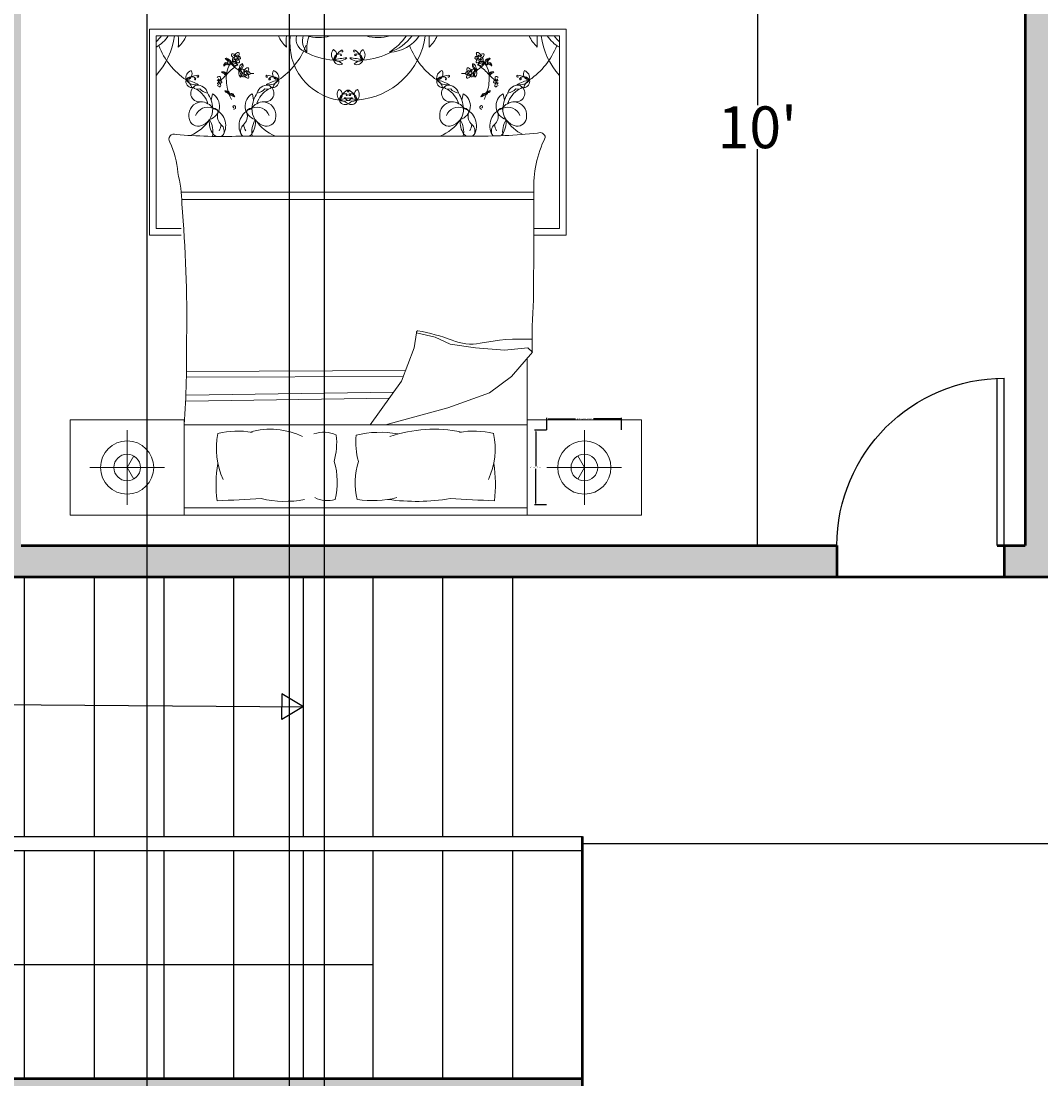
# Model space of a CAD drawing. Units: inches. Extents: x -22 to 470, y -437 to 97.
# Tile 6 of 9: x 88 to 235, y -192 to -41. Entities that reach past the tile are written whole.
import ezdxf

# ---------------------------------------------------------------- set-up
doc = ezdxf.new("R2010")
doc.units = ezdxf.units.IN
doc.header["$MEASUREMENT"] = 0
for name, color, linetype, lineweight in [('A-ANNO-DIMS', 2, 'Continuous', 18), ('A-DOOR', 4, 'Continuous', 25), ('A-FLOR-STRS', 7, 'Continuous', 25), ('A-FURN', 8, 'Continuous', 18), ('A-WALL', 7, 'Continuous', 50), ('A-WALL-PATT', 8, 'Continuous', 13)]:
    doc.layers.add(name, color=color, linetype=linetype, lineweight=lineweight)
doc.styles.get("Standard").update_dxf_attribs({"font": 'arial.ttf'})
doc.dimstyles.get("Standard").update_dxf_attribs({"dimtxt": 0.18, "dimasz": 0.18, "dimexe": 0.18, "dimexo": 0.0625, "dimgap": 0.09, "dimtad": 0, "dimtih": 1, "dimtoh": 1, "dimdec": 0, "dimzin": 0, "dimdsep": 46, "dimlunit": 3, "dimtxsty": 'Standard', "dimcen": 0.09, "dimadec": 0, "dimazin": 0, "dimtfac": 1, "dimtdec": 0, "dimtofl": 0, "dimtmove": 0, "dimatfit": 3, "dimfxl": 1, "dimtolj": 1, "dimtzin": 0, "dimarcsym": 0})

# ---------------------------------------------------------------- blocks, each defined once
blk = doc.blocks.new('*D6')
at = {"layer": 'A-ANNO-DIMS', "color": 0, "lineweight": -2, "transparency": 16777216}
for p, q in [((194.01, 4.06), (194.01, -52.6)), ((194.07, 4.24), (194.19, 4.24)), ((194.01, -115.58), (194.01, -58.91)), ((194.07, -115.76), (194.19, -115.76))]:
    blk.add_line(p, q, dxfattribs=at)
at = {"layer": 'A-ANNO-DIMS', "color": 0, "transparency": 16777216}
for points in [[(193.98, 4.06), (194.04, 4.06), (194.01, 4.24)], [(193.98, -115.58), (194.04, -115.58), (194.01, -115.76)]]:
    blk.add_solid(points, dxfattribs=at)
at = {"layer": 'Defpoints', "color": 0, "transparency": 16777216}
for p in [(194.01, 4.24), (194.01, 4.24), (194.01, -115.76)]:
    blk.add_point(p, dxfattribs=at)
at = {"layer": 'A-ANNO-DIMS', "color": 0, "transparency": 16777216, "insert": (194.01, -55.76), "char_height": 6, "attachment_point": 5}
blk.add_mtext("\\A1;10'", dxfattribs=at)
blk = doc.blocks.new('*D12')
at = {"layer": 'A-ANNO-DIMS', "color": 0, "lineweight": -2, "transparency": 16777216}
for p, q in [((168.92, -159.44), (168.92, -158.33)), ((169.1, -158.51), (240.81, -158.51)), ((332.74, -158.51), (261.03, -158.51)), ((332.92, -158.44), (332.92, -158.33))]:
    blk.add_line(p, q, dxfattribs=at)
at = {"layer": 'A-ANNO-DIMS', "color": 0, "transparency": 16777216}
for points in [[(169.1, -158.48), (169.1, -158.54), (168.92, -158.51)], [(332.74, -158.48), (332.74, -158.54), (332.92, -158.51)]]:
    blk.add_solid(points, dxfattribs=at)
at = {"layer": 'Defpoints', "color": 0, "transparency": 16777216}
for p in [(332.92, -158.51), (332.92, -158.51), (168.92, -159.51)]:
    blk.add_point(p, dxfattribs=at)
at = {"layer": 'A-ANNO-DIMS', "color": 0, "transparency": 16777216, "insert": (250.92, -158.51), "char_height": 6, "attachment_point": 5}
blk.add_mtext('\\A1;13\'-8"', dxfattribs=at)
blk = doc.blocks.new('DOOR-SWING-24')
for p, q in [((23, 24), (23, 0)), ((24, 24), (24, 0))]:
    blk.add_line(p, q)
blk.add_arc((24, 24), 24, 180, 270)
blk = doc.blocks.new('BEDSIDE-LAMP-LARGE')
for p, q in [((5.35, 10.71), (5.35, 0)), ((10.71, 5.36), (0, 5.36))]:
    blk.add_line(p, q)
for points in [[(5.35, 5.36), (6.31, 7.01)], [(5.35, 5.36), (6.31, 3.7)]]:
    blk.add_lwpolyline(points)
for radius in [3.82, 1.91]:
    blk.add_circle((5.35, 5.36), radius)
blk = doc.blocks.new('*D51')
at = {"layer": 'A-ANNO-DIMS', "color": 0, "lineweight": -2, "transparency": 16777216}
for p, q in [((163.84, -99.14), (163.84, -97.42)), ((164.02, -97.6), (167.91, -97.6)), ((174.37, -97.6), (170.49, -97.6)), ((174.55, -99.14), (174.55, -97.42))]:
    blk.add_line(p, q, dxfattribs=at)
at = {"layer": 'A-ANNO-DIMS', "color": 0, "transparency": 16777216}
for points in [[(164.02, -97.57), (164.02, -97.63), (163.84, -97.6)], [(174.37, -97.57), (174.37, -97.63), (174.55, -97.6)]]:
    blk.add_solid(points, dxfattribs=at)
at = {"layer": 'Defpoints', "color": 0, "transparency": 16777216}
for p in [(163.84, -97.6), (163.84, -99.21), (174.55, -99.21)]:
    blk.add_point(p, dxfattribs=at)
at = {"layer": 'A-ANNO-DIMS', "color": 0, "transparency": 16777216, "insert": (169.2, -97.6), "char_height": 0.18, "attachment_point": 5}
blk.add_mtext('\\A1;LAMP 0\'-10 1/2" TYP.', dxfattribs=at)
blk = doc.blocks.new('*D52')
at = {"layer": 'A-ANNO-DIMS', "color": 0, "lineweight": -2, "transparency": 16777216}
for p, q in [((163.78, -99.21), (162.06, -99.21)), ((162.24, -99.39), (162.24, -104.38)), ((162.24, -109.74), (162.24, -104.74)), ((163.78, -109.92), (162.06, -109.92))]:
    blk.add_line(p, q, dxfattribs=at)
at = {"layer": 'A-ANNO-DIMS', "color": 0, "transparency": 16777216}
for points in [[(162.21, -99.39), (162.27, -99.39), (162.24, -99.21)], [(162.21, -109.74), (162.27, -109.74), (162.24, -109.92)]]:
    blk.add_solid(points, dxfattribs=at)
at = {"layer": 'Defpoints', "color": 0, "transparency": 16777216}
for p in [(163.84, -99.21), (162.24, -109.92), (163.84, -109.92)]:
    blk.add_point(p, dxfattribs=at)
at = {"layer": 'A-ANNO-DIMS', "color": 0, "transparency": 16777216, "insert": (162.24, -104.56), "char_height": 0.18, "attachment_point": 5}
blk.add_mtext('\\A1;0\'-10 1/2" TYP.', dxfattribs=at)
blk = doc.blocks.new('*D79')
at = {"layer": 'A-ANNO-DIMS', "color": 0, "lineweight": -2, "transparency": 16777216}
for p, q in [((61.08, -228.48), (61.08, 40.87)), ((61.26, 40.69), (93.66, 40.69)), ((126.72, 40.69), (94.32, 40.69)), ((126.9, -228.48), (126.9, 40.87))]:
    blk.add_line(p, q, dxfattribs=at)
at = {"layer": 'A-ANNO-DIMS', "color": 0, "transparency": 16777216}
for points in [[(61.26, 40.72), (61.26, 40.66), (61.08, 40.69)], [(126.72, 40.72), (126.72, 40.66), (126.9, 40.69)]]:
    blk.add_solid(points, dxfattribs=at)
at = {"layer": 'Defpoints', "color": 0, "transparency": 16777216}
for p in [(126.9, 40.69), (61.08, -228.55), (126.9, -228.55)]:
    blk.add_point(p, dxfattribs=at)
at = {"layer": 'A-ANNO-DIMS', "color": 0, "transparency": 16777216, "insert": (93.99, 40.69), "char_height": 0.18, "attachment_point": 5}
blk.add_mtext('\\A1;5\'-6"', dxfattribs=at)
blk = doc.blocks.new('*D84')
at = {"layer": 'A-ANNO-DIMS', "color": 0, "lineweight": -2, "transparency": 16777216}
for p, q in [((106.48, -369.14), (106.48, 40.87)), ((106.66, 40.69), (118.66, 40.69)), ((131.74, 40.69), (119.74, 40.69)), ((131.92, -388.69), (131.92, 40.87))]:
    blk.add_line(p, q, dxfattribs=at)
at = {"layer": 'A-ANNO-DIMS', "color": 0, "transparency": 16777216}
for points in [[(106.66, 40.72), (106.66, 40.66), (106.48, 40.69)], [(131.74, 40.72), (131.74, 40.66), (131.92, 40.69)]]:
    blk.add_solid(points, dxfattribs=at)
at = {"layer": 'Defpoints', "color": 0, "transparency": 16777216}
for p in [(131.92, 40.69), (106.48, -369.2), (131.92, -388.76)]:
    blk.add_point(p, dxfattribs=at)
at = {"layer": 'A-ANNO-DIMS', "color": 0, "transparency": 16777216, "insert": (119.2, 40.69), "char_height": 0.18, "attachment_point": 5}
blk.add_mtext('\\A1;2\'-1 1/2"', dxfattribs=at)

msp = doc.modelspace()

# ---------------------------------------------------------------- hatches: boundary and pattern name
at = {"layer": 'A-WALL-PATT'}
h = msp.add_hatch(color=256, dxfattribs=at)
h.dxf.hatch_style = 1
h.paths.add_polyline_path([(130.42, 13.24), (26.92, 13.24), (26.92, -43.76), (35.92, -43.76), (35.92, 4.24), (83.92, 4.24), (83.92, 1.24), (88.42, 1.24), (88.42, 4.24), (130.42, 4.24)])
h.paths.add_polyline_path([(266.92, 13.24), (190.42, 13.24), (190.42, 4.24), (232.42, 4.24), (232.42, -115.76), (229.42, -115.76), (229.42, -120.26), (239.92, -120.26), (239.92, -115.76), (236.92, -115.76), (236.92, 4.24), (266.92, 4.24)])
h.paths.add_polyline_path([(442.42, 13.24), (326.92, 13.24), (326.92, 4.24), (356.92, 4.24), (356.92, 1.24), (361.42, 1.24), (361.42, 4.24), (433.42, 4.24), (433.42, -49.38), (442.42, -49.38)])
h.paths.add_polyline_path([(442.42, -73.38), (433.42, -73.38), (433.42, -115.76), (361.42, -115.76), (361.42, -22.76), (356.92, -22.76), (356.92, -115.76), (263.92, -115.76), (263.92, -120.26), (332.92, -120.26), (332.92, -123.26), (337.42, -123.26), (337.42, -120.26), (433.42, -120.26), (433.42, -148.49), (442.42, -148.49)])
h.paths.add_polyline_path([(205.42, -115.76), (88.42, -115.76), (88.42, -22.76), (83.92, -22.76), (83.92, -115.76), (35.92, -115.76), (35.92, -67.76), (26.92, -67.76), (26.92, -126.26), (35.92, -126.26), (35.92, -120.26), (205.42, -120.26)])
h.paths.add_polyline_path([(35.92, -196.76), (168.92, -196.76), (168.92, -192.26), (35.92, -192.26), (35.92, -186.26), (26.92, -186.26), (26.92, -224.25), (35.92, -224.25)])
h.paths.add_polyline_path([(35.92, -284.25), (26.92, -284.25), (26.92, -397.76), (53.92, -397.76), (53.92, -388.76), (35.92, -388.76)])
h.paths.add_polyline_path([(142.42, -388.76), (136.42, -388.76), (136.42, -316.76), (181.42, -316.76), (181.42, -312.26), (136.42, -312.26), (136.42, -303.75), (131.92, -303.75), (131.92, -388.76), (113.92, -388.76), (113.92, -397.76), (142.42, -397.76)])
h.paths.add_polyline_path([(218.92, -388.76), (212.92, -388.76), (212.92, -312.26), (205.42, -312.26), (205.42, -316.76), (208.42, -316.76), (208.42, -388.76), (202.42, -388.76), (202.42, -397.76), (218.92, -397.76)])
h.paths.add_polyline_path([(306.75, -388.76), (289.42, -388.76), (289.42, -316.76), (284.92, -316.76), (284.92, -388.76), (278.92, -388.76), (278.92, -397.76), (306.75, -397.76)])
h.paths.add_polyline_path([(391.42, -388.76), (366.75, -388.76), (366.75, -397.76), (391.42, -397.76)], flags=17)
h.paths.add_polyline_path([(442.42, -172.49), (433.42, -172.49), (433.42, -192.26), (337.42, -192.26), (337.42, -147.26), (332.92, -147.26), (332.92, -196.76), (433.42, -196.76), (433.42, -388.76), (427.42, -388.76), (427.42, -397.76), (442.42, -397.76)])

# ---------------------------------------------------------------- linework, layer by layer
at = {"layer": 'A-FLOR-STRS'}
for p, q in [((88.92, -157.51), (88.92, -120.26)), ((98.92, -157.51), (98.92, -120.26)), ((108.92, -157.51), (108.92, -120.26)), ((118.92, -157.51), (118.92, -120.26)), ((128.92, -157.51), (128.92, -120.26)), ((138.92, -157.51), (138.92, -120.26)), ((148.92, -157.51), (148.92, -120.26)), ((158.92, -157.51), (158.92, -120.26)), ((125.81, -137.02), (125.79, -138.86)), ((128.92, -138.88), (125.81, -137.02)), ((59.19, -138.35), (128.92, -138.88)), ((125.81, -140.69), (125.79, -138.86)), ((128.92, -138.83), (125.81, -140.69)), ((68.92, -157.51), (168.92, -157.51)), ((68.92, -159.51), (168.92, -159.51)), ((88.92, -192.26), (88.92, -159.51)), ((98.92, -192.26), (98.92, -159.51)), ((108.92, -192.26), (108.92, -159.51)), ((118.92, -192.26), (118.92, -159.51)), ((128.92, -192.26), (128.92, -159.51)), ((138.92, -192.26), (138.92, -159.51)), ((148.92, -192.26), (148.92, -159.51)), ((158.92, -192.26), (158.92, -159.51)), ((138.92, -175.88), (59.19, -175.88))]:
    msp.add_line(p, q, dxfattribs=at)
at = {"layer": 'A-FURN'}
for p, q in [((106.82, -41.69), (166.58, -41.69)), ((106.82, -71.21), (106.82, -41.69)), ((166.58, -41.69), (166.58, -71.21)), ((107.77, -42.64), (107.77, -70.26)), ((165.63, -42.64), (107.77, -42.64)), ((165.63, -70.26), (165.63, -42.64)), ((115.85, -50.95), (115.67, -51.87)), ((121.58, -50.95), (121.76, -51.87)), ((151.82, -50.95), (151.64, -51.87)), ((157.55, -50.95), (157.73, -51.87)), ((119.77, -57.03), (153.05, -57.03)), ((111.37, -65.08), (161.95, -65.08)), ((111.45, -66.1), (161.95, -66.1)), ((111.37, -71.21), (106.82, -71.21)), ((107.77, -70.26), (111.39, -70.26)), ((161.94, -70.26), (165.63, -70.26)), ((166.58, -71.21), (161.94, -71.21)), ((144.8, -87.38), (145.14, -85.22)), ((145.14, -85.22), (147.79, -85.88)), ((147.79, -85.88), (149.95, -86.88)), ((142.98, -92.19), (144.8, -87.38)), ((149.95, -86.88), (153.6, -87.38)), ((153.6, -87.38), (157.75, -87.71)), ((157.75, -87.71), (161.07, -87.38)), ((161.07, -87.38), (161.74, -88.04)), ((161.74, -88.04), (158.75, -91.52)), ((161, -111.39), (161, -88.89)), ((112.11, -90.77), (143.56, -90.64)), ((112.12, -91.61), (143.24, -91.49)), ((138.49, -98.44), (142.98, -92.19)), ((158.75, -91.52), (155.59, -93.85)), ((112.08, -94.19), (141.84, -93.77)), ((155.59, -93.85), (149.62, -96)), ((112.04, -95.03), (141.23, -94.62)), ((149.62, -96), (140.68, -98.44)), ((161, -98.44), (111.82, -98.44)), ((111.82, -110.34), (161, -110.34)), ((177.4, -111.39), (95.43, -111.39))]:
    msp.add_line(p, q, dxfattribs=at)
for points in [[(161.91, -80.53, 0.001242), (161.95, -64.98, -0.127202), (163.59, -57.23)], [(111.48, -66.75, 0.056112), (110.88, -62.24, 0.095341), (109.73, -57.89)], [(116.53, -109.35, -0.074897), (116.63, -103.99, 0.472817)], [(133.3, -103.7, -0.14099), (133.46, -109.16, -0.235245)], [(136.8, -103.7, 0.14099), (136.63, -109.16, 0.235245)], [(156.3, -109.35, 0.074897), (156.2, -103.99, -0.472817)]]:
    msp.add_lwpolyline(points, format="xyb", dxfattribs=at)
for points in [[(111.82, -111.39), (111.82, -97.73), (95.43, -97.73), (95.43, -111.39)], [(161, -97.73), (177.4, -97.73), (177.4, -111.39)]]:
    msp.add_lwpolyline(points, dxfattribs=at)
for centre in [(119.22, -45.78), (154.18, -45.78), (120.58, -47.98), (152.82, -47.98)]:
    msp.add_circle(centre, 0.209, dxfattribs=at)
for centre, radius, start, end in [((105.17, -39.76), 5.22, 299.8884, 326.5383), ((103.3, -38.79), 6.5, 313.5186, 323.6964), ((99.8, -41.19), 10.7, 318.1144, 352.255), ((108.09, -40.97), 4.35, 311.0454, 337.4453), ((96.17, -43.31), 14.81, 356.3481, 2.5919), ((129.33, -40.97), 4.35, 202.5547, 228.9546), ((141.25, -43.31), 14.81, 177.4081, 183.6519), ((135.24, -43.67), 8.28, 172.8636, 261.8197), ((129.77, -43.09), 1.92, 166.3898, 259.0739), ((131.21, -43.35), 2.43, 162.8609, 221.9049), ((131.08, -37.01), 5.89, 252.9798, 286.4569), ((134.17, -44.42), 4.79, 158.117, 186.6195), ((133.41, -33.98), 8.7, 264.3643, 265.6213), ((137.99, -28.01), 15.55, 250.0972, 250.2783), ((135.78, -41.19), 10.7, 274.4623, 352.255), ((139.59, -37.01), 5.89, 253.5431, 287.0202), ((137.26, -33.98), 8.7, 274.3787, 275.6357), ((132.67, -28.01), 15.55, 289.7217, 289.9028), ((141.15, -39.76), 5.22, 271.272, 326.5383), ((135.85, -36.96), 9.67, 304.0123, 324.053), ((139.27, -38.79), 6.5, 287.8504, 323.6964), ((132.15, -43.31), 14.81, 356.3481, 2.5919), ((144.07, -40.97), 4.35, 311.0454, 337.4453), ((165.31, -40.97), 4.35, 202.5547, 228.9546), ((177.23, -43.31), 14.81, 177.4081, 183.6519), ((173.6, -41.19), 10.7, 187.745, 221.8856), ((168.23, -39.76), 5.22, 213.4617, 240.1116), ((170.1, -38.79), 6.5, 216.3036, 226.4814), ((118.12, -40.14), 10.7, 201.4092, 235.6135), ((118.78, -45.38), 0.207, 134.3732, 211.9501), ((119.16, -45.15), 0.658, 211.9501, 255.2442), ((118.79, -45.62), 0.412, 8.5614, 112.5914), ((118.91, -45.6), 0.138, 352.868, 97.094), ((119.5, -45.39), 0.345, 100.9597, 208.7804), ((119.88, -45.85), 0.634, 132.3896, 156.5724), ((119.21, -45.21), 0.485, 291.6382, 4.947), ((119.54, -45.18), 0.16, 4.947, 127.5263), ((119.31, -40.14), 10.7, 304.3865, 338.5908), ((134.07, -35.46), 10.7, 242.5854, 265.5377), ((134.12, -45.34), 1.19, 140.8855, 222.2127), ((132.77, -45.37), 0.894, 301.6373, 61.4609), ((135.8, -47.01), 2.71, 121.989, 161.0841), ((134.11, -46.1), 0.876, 76.148, 182.2415), ((134.31, -45.41), 0.0698, 140.1909, 76.0209), ((134.44, -44.83), 0.133, 288.4408, 121.989), ((134.46, -44.89), 0.0646, 171.9833, 288.4408), ((136.23, -44.83), 0.133, 58.011, 251.5592), ((136.21, -44.89), 0.0646, 251.5592, 8.0167), ((136.37, -45.36), 0.116, 103.852, 39.9245), ((134.87, -47.01), 2.71, 18.9159, 58.011), ((136.55, -46.1), 0.876, 357.7585, 103.852), ((137.9, -45.37), 0.894, 118.5391, 238.3627), ((136.55, -45.34), 1.19, 317.7873, 39.1145), ((136.6, -35.46), 10.7, 274.4623, 297.4146), ((154.09, -40.14), 10.7, 201.4092, 235.6135), ((153.86, -45.18), 0.16, 52.4737, 175.053), ((154.19, -45.21), 0.485, 175.053, 248.3618), ((153.52, -45.85), 0.634, 23.4276, 47.6104), ((153.9, -45.39), 0.345, 331.2196, 79.0403), ((154.61, -45.62), 0.412, 67.4086, 171.4386), ((154.49, -45.6), 0.138, 82.906, 187.132), ((154.24, -45.15), 0.658, 284.7558, 328.0499), ((154.62, -45.38), 0.207, 328.0499, 45.6268), ((155.28, -40.14), 10.7, 304.3865, 338.5908), ((117.7, -46.84), 0.233, 123.0979, 213.1364), ((118.1, -47.18), 0.631, 92.3172, 160.5201), ((120.99, -51.98), 6.1, 121.1156, 124.8118), ((118.03, -46.94), 0.543, 82.6008, 147.1845), ((117.87, -46.08), 0.233, 55.6077, 145.6462), ((117.71, -46.58), 0.631, 21.7087, 93.0299), ((114.39, -51.08), 6.1, 53.6254, 57.3216), ((117.96, -46.96), 0.241, 45.7354, 121.1156), ((121.25, -48.5), 3.4, 150.7959, 175.244), ((126.15, -55.75), 11.2, 127.8256, 137.7588), ((117.91, -46.42), 0.543, 342.8042, 79.6943), ((117.86, -46.37), 0.241, 338.2452, 53.6254), ((118.25, -46.52), 0.182, 158.2452, 340.6395), ((118.26, -46.66), 0.182, 225.7354, 48.1297), ((121.68, -45), 3.64, 201.7087, 206.2181), ((118.78, -47.48), 0.951, 40.9365, 112.7695), ((118.47, -47.16), 0.56, 49.3812, 95.5456), ((121.25, -48.5), 3.4, 137.5083, 145.9967), ((118.88, -46.94), 0.578, 61.1838, 141.6792), ((121.6, -43.98), 4.08, 220.182, 239.456), ((118.99, -46.07), 0.285, 88.5719, 233.8954), ((118.96, -46.14), 0.205, 228.2946, 6.2474), ((119.27, -46.23), 0.673, 229.3812, 289.9959), ((118.76, -45.9), 0.287, 298.8493, 359.9355), ((118.83, -46.15), 0.328, 4.2123, 48.1587), ((119.51, -46.1), 0.348, 183.635, 258.4363), ((118.84, -47.05), 0.691, 15.6484, 62.2957), ((119.46, -45.97), 0.199, 178.1325, 268.8919), ((119.6, -45.93), 0.342, 42.3208, 130.2111), ((119.67, -45.57), 0.432, 226.3462, 279.6513), ((119.23, -46.37), 0.502, 7.4968, 71.2737), ((119.59, -45.12), 0.683, 254.2829, 276.9148), ((119.57, -46.35), 0.161, 215.0752, 14.7644), ((119.23, -46.6), 0.951, 287.889, 359.722), ((119.72, -45.82), 0.18, 279.6513, 42.3208), ((120.42, -47.23), 0.673, 110.6625, 171.2773), ((119.56, -46.89), 0.691, 338.3627, 25.0101), ((135.48, -53.28), 7.49, 92.7418, 107.407), ((133.94, -44.59), 1.69, 245.6899, 314.4589), ((133.19, -47.96), 1.83, 44.6273, 88.5415), ((134.09, -45.89), 0.887, 196.1963, 296.9726), ((135.19, -53.28), 7.49, 72.593, 87.2582), ((136.73, -44.59), 1.69, 225.5411, 294.3101), ((137.48, -47.96), 1.83, 91.4585, 135.3727), ((136.58, -45.89), 0.887, 243.0274, 343.8037), ((153.84, -46.89), 0.691, 154.9899, 201.6373), ((154.17, -46.6), 0.951, 180.278, 252.111), ((152.98, -47.23), 0.673, 8.7227, 69.3375), ((153.68, -45.82), 0.18, 137.6792, 260.3487), ((153.8, -45.93), 0.342, 49.7889, 137.6792), ((153.73, -45.57), 0.432, 260.3487, 313.6538), ((154.17, -46.37), 0.502, 108.7263, 172.5032), ((153.83, -46.35), 0.161, 165.2356, 324.9248), ((153.81, -45.12), 0.683, 263.0852, 285.7171), ((151.8, -43.98), 4.08, 300.544, 319.818), ((154.56, -47.05), 0.691, 117.7043, 164.3516), ((154.62, -47.48), 0.951, 67.2305, 139.0635), ((154.13, -46.23), 0.673, 250.0041, 310.6188), ((153.94, -45.97), 0.199, 271.1081, 1.8675), ((153.89, -46.1), 0.348, 281.5637, 356.365), ((147.25, -55.75), 11.2, 42.2412, 52.1744), ((154.57, -46.15), 0.328, 131.8413, 175.7877), ((154.44, -46.14), 0.205, 173.7526, 311.7054), ((154.52, -46.94), 0.578, 38.3208, 118.8162), ((154.63, -45.9), 0.287, 180.0645, 241.1507), ((154.41, -46.07), 0.285, 306.1046, 91.4281), ((154.93, -47.16), 0.56, 84.4544, 130.6188), ((152.15, -48.5), 3.4, 34.0033, 42.4917), ((155.49, -46.42), 0.543, 100.3057, 197.1958), ((155.14, -46.66), 0.182, 131.8703, 314.2646), ((155.14, -46.52), 0.182, 199.3605, 21.7548), ((151.72, -45), 3.64, 333.7819, 338.2913), ((155.69, -46.58), 0.631, 86.9701, 158.2913), ((152.15, -48.5), 3.4, 4.756, 29.2041), ((155.44, -46.96), 0.241, 58.8844, 134.2646), ((155.54, -46.37), 0.241, 126.3746, 201.7548), ((155.37, -46.94), 0.543, 32.8155, 97.3992), ((155.3, -47.18), 0.631, 19.4799, 87.6828), ((155.53, -46.08), 0.233, 34.3538, 124.3923), ((159.01, -51.08), 6.1, 122.6784, 126.3746), ((152.41, -51.98), 6.1, 55.1882, 58.8844), ((155.7, -46.84), 0.233, 326.8636, 56.9021), ((113.23, -48.72), 1.19, 110.9613, 192.2885), ((112.04, -48.08), 0.894, 271.7131, 31.5367), ((113.85, -51.01), 2.71, 92.0648, 131.1598), ((112.85, -49.38), 0.876, 46.2238, 152.3173), ((113.75, -48.5), 0.0646, 142.0591, 258.5166), ((113.76, -48.43), 0.133, 258.5166, 92.0648), ((116.82, -48.83), 0.345, 100.9597, 142.2379), ((116.85, -48.62), 0.16, 4.947, 127.5263), ((112.18, -42.9), 7.78, 307.9541, 316.8459), ((117.23, -50.09), 2.31, 82.8698, 91.6736), ((117.56, -47.6), 0.43, 205.5379, 258.6744), ((116.94, -49.06), 1.3, 59.344, 79.7412), ((116.66, -49.05), 1.32, 43.6929, 51.7899), ((117.46, -48.19), 0.393, 355.7131, 81.6568), ((117.25, -48.53), 0.687, 27.3659, 59.344), ((117.76, -48.08), 0.167, 202.5583, 304.2343), ((124.63, -48.67), 6.79, 176.1723, 196.4158), ((119.49, -48.07), 0.578, 3.8774, 87.1501), ((119.2, -47.04), 0.56, 305.1128, 351.2773), ((119.09, -47.85), 0.56, 352.0748, 38.2393), ((118.99, -48.29), 0.951, 343.6301, 55.4631), ((120.31, -48.02), 0.673, 172.0748, 232.6895), ((119.66, -46.95), 0.578, 271.4625, 339.4747), ((119.38, -48.1), 0.691, 318.342, 4.9894), ((120.15, -47.58), 0.207, 134.3732, 211.9501), ((121.6, -43.98), 4.08, 246.1523, 246.9499), ((120.53, -47.35), 0.658, 211.9501, 255.2442), ((120.16, -47.82), 0.412, 8.5614, 112.5914), ((120.35, -48.27), 0.285, 88.5719, 233.8954), ((120.32, -48.34), 0.205, 228.2946, 6.2474), ((120.28, -47.8), 0.138, 352.868, 97.094), ((120.13, -48.1), 0.287, 298.8493, 359.9355), ((120.2, -48.35), 0.328, 4.2123, 48.1587), ((120.87, -47.59), 0.345, 100.9597, 208.7804), ((120.87, -48.3), 0.348, 183.635, 258.4363), ((120.83, -48.17), 0.199, 178.1325, 268.8919), ((121.24, -48.05), 0.634, 132.3896, 156.5724), ((120.96, -48.13), 0.342, 42.3208, 130.2111), ((121.04, -47.77), 0.432, 226.3462, 279.6513), ((120.59, -48.57), 0.502, 7.4968, 71.2737), ((120.58, -47.41), 0.485, 291.6382, 4.947), ((120.96, -47.32), 0.683, 254.2829, 276.9148), ((120.9, -47.38), 0.16, 4.947, 127.5263), ((120.94, -48.55), 0.161, 215.0752, 14.7644), ((121.08, -48.02), 0.18, 279.6513, 42.3208), ((121.6, -43.98), 4.08, 265.2415, 272.8929), ((123.67, -48.43), 0.133, 87.9352, 281.4834), ((123.57, -51.01), 2.71, 48.8402, 87.9352), ((123.68, -48.5), 0.0646, 281.4834, 37.9409), ((124.58, -49.38), 0.876, 27.6827, 133.7762), ((125.38, -48.08), 0.894, 148.4633, 268.2869), ((124.2, -48.72), 1.19, 347.7115, 69.0387), ((149.2, -48.72), 1.19, 110.9613, 192.2885), ((148.02, -48.08), 0.894, 271.7131, 31.5367), ((149.82, -51.01), 2.71, 92.0648, 131.1598), ((148.82, -49.38), 0.876, 46.2238, 152.3173), ((149.72, -48.5), 0.0646, 142.0591, 258.5166), ((149.73, -48.43), 0.133, 258.5166, 92.0648), ((151.8, -43.98), 4.08, 267.1071, 274.7585), ((152.32, -48.02), 0.18, 137.6792, 260.3487), ((152.44, -48.13), 0.342, 49.7889, 137.6792), ((152.36, -47.77), 0.432, 260.3487, 313.6538), ((152.46, -48.55), 0.161, 165.2356, 324.9248), ((152.81, -48.57), 0.502, 108.7263, 172.5032), ((152.5, -47.38), 0.16, 52.4737, 175.053), ((152.82, -47.41), 0.485, 175.053, 248.3618), ((152.44, -47.32), 0.683, 263.0852, 285.7171), ((152.57, -48.17), 0.199, 271.1081, 1.8675), ((152.16, -48.05), 0.634, 23.4276, 47.6104), ((152.53, -47.59), 0.345, 331.2196, 79.0403), ((152.53, -48.3), 0.348, 281.5637, 356.365), ((153.24, -47.82), 0.412, 67.4086, 171.4386), ((153.2, -48.35), 0.328, 131.8413, 175.7877), ((153.08, -48.34), 0.205, 173.7526, 311.7054), ((153.27, -48.1), 0.287, 180.0645, 241.1507), ((153.12, -47.8), 0.138, 82.906, 187.132), ((152.87, -47.35), 0.658, 284.7558, 328.0499), ((153.05, -48.27), 0.285, 306.1046, 91.4281), ((153.74, -46.95), 0.578, 200.5253, 268.5375), ((153.9, -48.07), 0.578, 92.8499, 176.1226), ((154.02, -48.1), 0.691, 175.0106, 221.658), ((153.25, -47.58), 0.207, 328.0499, 45.6268), ((151.8, -43.98), 4.08, 293.0501, 293.8477), ((154.41, -48.29), 0.951, 124.5369, 196.3699), ((153.09, -48.02), 0.673, 307.3105, 7.9252), ((154.2, -47.04), 0.56, 188.7227, 234.8872), ((154.31, -47.85), 0.56, 141.7607, 187.9252), ((148.77, -48.67), 6.79, 343.5842, 3.8277), ((155.94, -48.19), 0.393, 98.3432, 184.2869), ((156.15, -48.53), 0.687, 120.656, 152.6341), ((155.64, -48.08), 0.167, 235.7657, 337.4417), ((161.22, -42.9), 7.78, 223.1541, 232.0459), ((156.74, -49.05), 1.32, 128.2101, 136.3071), ((156.46, -49.06), 1.3, 100.2588, 120.656), ((156.17, -50.09), 2.31, 88.3264, 97.1302), ((155.84, -47.6), 0.43, 281.3256, 334.4621), ((156.55, -48.62), 0.16, 52.4737, 175.053), ((156.58, -48.83), 0.345, 37.7621, 79.0403), ((159.64, -48.43), 0.133, 87.9352, 281.4834), ((159.55, -51.01), 2.71, 48.8402, 87.9352), ((159.65, -48.5), 0.0646, 281.4834, 37.9409), ((160.55, -49.38), 0.876, 27.6827, 133.7762), ((161.36, -48.08), 0.894, 148.4633, 268.2869), ((160.17, -48.72), 1.19, 347.7115, 69.0387), ((112.93, -49.18), 0.887, 166.272, 267.0484), ((110.45, -56.28), 7.49, 62.8176, 77.4827), ((113.44, -47.98), 1.69, 215.7657, 284.5347), ((111.12, -50.53), 1.83, 14.7031, 58.6173), ((113.97, -50.88), 1.23, 109.1312, 279.736), ((113.72, -49.55), 0.754, 216.7319, 296.0245), ((113.36, -48.87), 0.0698, 110.2667, 46.2271), ((113.68, -51.25), 1.54, 15.6955, 94.031), ((116.54, -49.22), 0.209, 273.2768, 86.7232), ((116.83, -49.54), 0.348, 217.3642, 258.4363), ((116.78, -49.41), 0.199, 178.1325, 268.8919), ((117.19, -49.29), 0.634, 132.3896, 156.5724), ((116.92, -49.37), 0.342, 42.3208, 130.2111), ((116.99, -49.01), 0.432, 226.3462, 279.6513), ((116.53, -48.65), 0.485, 291.6382, 4.947), ((116.55, -49.81), 0.502, 7.4968, 71.2737), ((116.91, -48.57), 0.683, 254.2829, 276.9148), ((116.89, -49.79), 0.161, 215.0752, 14.7644), ((117.04, -49.26), 0.18, 279.6513, 42.3208), ((123.75, -51.25), 1.54, 85.969, 164.3045), ((123.45, -50.88), 1.23, 260.264, 70.8688), ((123.71, -49.55), 0.754, 243.9755, 323.2681), ((123.98, -47.98), 1.69, 255.4653, 324.2343), ((126.98, -56.28), 7.49, 102.5173, 117.1824), ((124.06, -48.83), 0.116, 133.7762, 69.7183), ((124.49, -49.18), 0.887, 272.9516, 13.728), ((126.31, -50.53), 1.83, 121.3827, 165.2969), ((148.91, -49.18), 0.887, 166.272, 267.0484), ((147.09, -50.53), 1.83, 14.7031, 58.6173), ((149.42, -47.98), 1.69, 215.7657, 284.5347), ((146.42, -56.28), 7.49, 62.8176, 77.4827), ((149.95, -50.88), 1.23, 109.1312, 279.736), ((149.69, -49.55), 0.754, 216.7319, 296.0245), ((149.33, -48.87), 0.0698, 110.2667, 46.2271), ((149.65, -51.25), 1.54, 15.6955, 94.031), ((156.36, -49.26), 0.18, 137.6792, 260.3487), ((156.48, -49.37), 0.342, 49.7889, 137.6792), ((156.41, -49.01), 0.432, 260.3487, 313.6538), ((156.85, -49.81), 0.502, 108.7263, 172.5032), ((156.51, -49.79), 0.161, 165.2356, 324.9248), ((156.87, -48.65), 0.485, 175.053, 248.3618), ((156.49, -48.57), 0.683, 263.0852, 285.7171), ((156.62, -49.41), 0.199, 271.1081, 1.8675), ((156.21, -49.29), 0.634, 23.4276, 47.6104), ((156.57, -49.54), 0.348, 281.5637, 322.6358), ((156.86, -49.22), 0.209, 93.2768, 266.7232), ((159.72, -51.25), 1.54, 85.969, 164.3045), ((159.42, -50.88), 1.23, 260.264, 70.8688), ((159.68, -49.55), 0.754, 243.9755, 323.2681), ((162.95, -56.28), 7.49, 102.5173, 117.1824), ((159.96, -47.98), 1.69, 255.4653, 324.2343), ((160.03, -48.83), 0.116, 133.7762, 69.7183), ((162.28, -50.53), 1.83, 121.3827, 165.2969), ((160.47, -49.18), 0.887, 272.9516, 13.728), ((111.54, -53.59), 3.87, 18.2955, 58.7386), ((115.33, -49.21), 1.64, 218.4175, 263.8338), ((111.5, -53.28), 4.4, 3.4924, 33.7117), ((114.83, -52.71), 2.04, 286.8663, 60.0915), ((117.72, -52.85), 2.31, 82.8698, 91.6736), ((118.04, -50.36), 0.43, 205.5379, 258.6744), ((117.42, -51.82), 1.3, 59.344, 79.7412), ((117.14, -51.81), 1.32, 43.6929, 51.7899), ((117.95, -50.95), 0.393, 355.7131, 81.6568), ((117.73, -51.29), 0.687, 27.3659, 59.344), ((118.25, -50.84), 0.167, 202.5583, 304.2343), ((124.63, -48.67), 6.79, 200.1059, 206.9968), ((118.56, -51.31), 0.393, 36.5232, 122.4668), ((118.35, -51.66), 0.687, 58.836, 90.8141), ((118.51, -50.99), 0.167, 173.9457, 275.6216), ((118.18, -52.43), 1.32, 66.3901, 74.4871), ((119.03, -50.95), 0.43, 219.5056, 272.6421), ((118.04, -52.18), 1.3, 38.4388, 58.836), ((116.99, -52.41), 2.31, 26.5064, 35.3102), ((122.59, -52.71), 2.04, 119.9085, 253.1337), ((125.93, -53.28), 4.4, 146.2883, 176.5076), ((125.89, -53.59), 3.87, 121.2614, 161.7045), ((122.09, -49.21), 1.64, 276.1662, 321.5825), ((134.94, -51.07), 1.19, 140.8855, 222.2127), ((133.59, -51.1), 0.894, 301.6373, 61.4609), ((136.62, -52.74), 2.71, 121.989, 161.0841), ((134.93, -51.83), 0.876, 76.148, 182.2415), ((134.75, -50.32), 1.69, 245.6899, 314.4589), ((136.3, -59.01), 7.49, 92.7418, 107.407), ((135.91, -50.32), 1.69, 225.5411, 294.3101), ((134.37, -59.01), 7.49, 72.593, 87.2582), ((135.13, -51.14), 0.0698, 140.1909, 76.0209), ((135.26, -50.56), 0.133, 288.4408, 121.989), ((135.28, -50.62), 0.0646, 171.9833, 288.4408), ((135.41, -50.56), 0.133, 58.011, 251.5592), ((135.39, -50.62), 0.0646, 251.5592, 8.0167), ((135.55, -51.09), 0.116, 103.852, 39.9245), ((134.05, -52.74), 2.71, 18.9159, 58.011), ((135.73, -51.83), 0.876, 357.7585, 103.852), ((137.08, -51.1), 0.894, 118.5391, 238.3627), ((135.73, -51.07), 1.19, 317.7873, 39.1145), ((147.51, -53.59), 3.87, 18.2955, 58.7386), ((151.31, -49.21), 1.64, 218.4175, 263.8338), ((147.47, -53.28), 4.4, 3.4924, 33.7117), ((150.81, -52.71), 2.04, 286.8663, 60.0915), ((156.41, -52.41), 2.31, 144.6898, 153.4936), ((155.36, -52.18), 1.3, 121.164, 141.5612), ((154.37, -50.95), 0.43, 267.3579, 320.4944), ((154.84, -51.31), 0.393, 57.5332, 143.4768), ((155.04, -51.66), 0.687, 89.1859, 121.164), ((155.22, -52.43), 1.32, 105.5129, 113.6099), ((148.77, -48.67), 6.79, 333.0032, 339.8941), ((154.89, -50.99), 0.167, 264.3784, 6.0543), ((155.45, -50.95), 0.393, 98.3432, 184.2869), ((155.66, -51.29), 0.687, 120.656, 152.6341), ((155.15, -50.84), 0.167, 235.7657, 337.4417), ((156.26, -51.81), 1.32, 128.2101, 136.3071), ((155.98, -51.82), 1.3, 100.2588, 120.656), ((155.68, -52.85), 2.31, 88.3264, 97.1302), ((155.36, -50.36), 0.43, 281.3256, 334.4621), ((158.57, -52.71), 2.04, 119.9085, 253.1337), ((161.9, -53.28), 4.4, 146.2883, 176.5076), ((161.86, -53.59), 3.87, 121.2614, 161.7045), ((158.07, -49.21), 1.64, 276.1662, 321.5825), ((114.43, -54.04), 1.96, 97.1143, 185.0551), ((115.2, -54.78), 1.9, 68.5779, 158.4181), ((113.43, -53.21), 2.47, 283.079, 4.7067), ((114.08, -54.47), 2.38, 35.9599, 87.6409), ((118.56, -54.95), 3.16, 143.6555, 147.2989), ((116.12, -53.57), 0.509, 344.8529, 102.6959), ((115.15, -55.54), 2.61, 330.8249, 70.7178), ((118.95, -52.8), 0.158, 79.5616, 257.2949), ((118.93, -52.9), 0.257, 259.5864, 79.5616), ((122.28, -55.54), 2.61, 109.2822, 209.1751), ((121.3, -53.57), 0.509, 77.3041, 195.1471), ((123.34, -54.47), 2.38, 92.3591, 144.0401), ((118.87, -54.95), 3.16, 32.7011, 36.3445), ((123.99, -53.21), 2.47, 175.2933, 256.921), ((122.23, -54.78), 1.9, 21.5819, 111.4221), ((123, -54.04), 1.96, 354.9449, 82.8857), ((134.91, -51.62), 0.887, 196.1963, 296.9726), ((134.01, -53.69), 1.83, 44.6273, 88.5415), ((135.76, -51.62), 0.887, 243.0274, 343.8037), ((136.66, -53.69), 1.83, 91.4585, 135.3727), ((150.4, -54.04), 1.96, 97.1143, 185.0551), ((151.17, -54.78), 1.9, 68.5779, 158.4181), ((149.41, -53.21), 2.47, 283.079, 4.7067), ((150.06, -54.47), 2.38, 35.9599, 87.6409), ((154.53, -54.95), 3.16, 143.6555, 147.2989), ((152.1, -53.57), 0.509, 344.8529, 102.6959), ((151.12, -55.54), 2.61, 330.8249, 70.7178), ((154.47, -52.9), 0.257, 100.4384, 280.4136), ((154.45, -52.8), 0.158, 282.7051, 100.4384), ((158.25, -55.54), 2.61, 109.2822, 209.1751), ((157.28, -53.57), 0.509, 77.3041, 195.1471), ((159.31, -54.47), 2.38, 92.3591, 144.0401), ((154.84, -54.95), 3.16, 32.7011, 36.3445), ((159.97, -53.21), 2.47, 175.2933, 256.921), ((158.2, -54.78), 1.9, 21.5819, 111.4221), ((158.97, -54.04), 1.96, 354.9449, 82.8857), ((113.86, -54.23), 1.38, 178.9462, 275.5144), ((118.24, -54.14), 1.68, 164.8529, 228.4347), ((119.19, -54.14), 1.68, 311.5653, 15.1471), ((123.57, -54.23), 1.38, 264.4856, 1.0538), ((149.83, -54.23), 1.38, 178.9462, 275.5144), ((154.21, -54.14), 1.68, 164.8529, 228.4347), ((155.16, -54.14), 1.68, 311.5653, 15.1471), ((159.54, -54.23), 1.38, 264.4856, 1.0538), ((110.24, -51.26), 6.2, 293.6453, 326.3329), ((118.56, -54.95), 3.16, 175.2696, 214.215), ((112.52, -56.42), 3.4, 349.249, 31.1782), ((114.76, -55.07), 2.36, 330.0851, 352.564), ((116.31, -56.32), 1.23, 336.1646, 48.4347), ((121.12, -56.32), 1.23, 131.5653, 203.8354), ((122.67, -55.07), 2.36, 187.436, 209.9149), ((118.87, -54.95), 3.16, 325.785, 4.7304), ((124.91, -56.42), 3.4, 148.8218, 190.2867), ((127.18, -51.26), 6.2, 213.6671, 248.5059), ((146.22, -51.26), 6.2, 291.4941, 326.3329), ((154.53, -54.95), 3.16, 175.2696, 214.215), ((148.49, -56.42), 3.4, 349.7133, 31.1782), ((150.73, -55.07), 2.36, 330.0851, 352.564), ((152.28, -56.32), 1.23, 336.1646, 48.4347), ((157.09, -56.32), 1.23, 131.5653, 203.8354), ((158.64, -55.07), 2.36, 187.436, 209.9149), ((154.84, -54.95), 3.16, 325.785, 4.7304), ((160.88, -56.42), 3.4, 148.8218, 189.1554), ((163.16, -51.26), 6.2, 213.6671, 243.2997), ((110.35, -57.48), 0.747, 66.5219, 213.8264), ((117.26, 22.69), 79.76, 265.2402, 271.8035), ((116.73, -56.12), 0.987, 217.675, 252.5814), ((116.73, -56.12), 0.987, 286.6343, 315.5483), ((120.7, -56.12), 0.987, 224.4517, 246.7144), ((120.7, -56.12), 0.987, 293.2856, 322.325), ((152.7, -56.12), 0.987, 217.675, 246.7144), ((154.03, 28.29), 85.32, 269.3433, 275.6887), ((152.7, -56.12), 0.987, 293.229, 315.5483), ((156.67, -56.12), 0.987, 224.4517, 243.558), ((156.67, -56.12), 0.987, 300.0293, 322.325), ((162.84, -57.28), 0.756, 3.98, 117.3412), ((-79.94, -83.07), 192.11, 359.1145, 4.8735), ((236.89, -86), 75.18, 175.8294, 181.553), ((145.32, -85.15), 0.198, 88.8623, 199.7536), ((139.44, -116.19), 31.79, 70.1194, 79.3383), ((-35.11, -88.42), 147.27, 356.1, 0.9282), ((152.94, -80.19), 6.67, 246.2616, 281.3392), ((160.33, -117.06), 30.93, 87.4519, 101.3392), ((126.97, -101.85), 10.56, 168.2417, 204.8684), ((119.46, -110.31), 10.98, 78.9631, 104.8961), ((124.2, -109.5), 10.43, 63.8761, 106.1746), ((131.79, -103.85), 4.35, 65.0183, 108.5407), ((123.64, -100.96), 10.04, 344.1707, 5.9871), ((146.46, -100.96), 10.04, 174.0129, 195.8293), ((139.88, -113.96), 14.45, 79.8617, 103.6238), ((147.59, -118.12), 19.05, 78.0397, 109.2615), ((153.37, -110.31), 10.98, 75.1039, 101.0369), ((145.85, -101.85), 10.56, 335.1316, 11.7583), ((161.71, -889.37), 781.32, 92.85022, 93.31479), ((126.26, -95.01), 14.41, 256.3427, 281.1841), ((132.34, -105.26), 4.05, 243.3437, 286.1026), ((138.79, -94.71), 14.6, 261.5249, 283.96), ((145.06, -79.69), 29.73, 262.2196, 279.497), ((111.12, -889.37), 781.32, 86.68521, 87.14978)]:
    msp.add_arc(centre, radius, start, end, dxfattribs=at)
at = {"layer": 'A-WALL'}
for p, q in [((232.42, 4.24), (232.42, -115.76)), ((88.42, -115.76), (205.42, -115.76)), ((205.42, -115.76), (205.42, -120.26)), ((228.42, -115.76), (232.42, -115.76)), ((229.42, -115.76), (229.42, -120.26)), ((35.92, -120.26), (332.92, -120.26)), ((168.92, -196.76), (168.92, -157.51)), ((168.92, -192.26), (35.92, -192.26))]:
    msp.add_line(p, q, dxfattribs=at)

# ---------------------------------------------------------------- block references
at = {"layer": 'A-DOOR', "extrusion": (0, 0, -1), "zscale": -1, "rotation": 180}
msp.add_blockref('DOOR-SWING-24', (-205.42, -91.76), dxfattribs=at)
at = {"layer": 'A-FURN'}
msp.add_blockref('BEDSIDE-LAMP-LARGE', (98.27, -109.92), dxfattribs=at)
at = {"layer": 'A-FURN', "rotation": 180}
msp.add_blockref('BEDSIDE-LAMP-LARGE', (174.55, -99.21), dxfattribs=at)

# ---------------------------------------------------------------- dimensions: what is measured, and where the dimension line sits
at = {"layer": 'A-ANNO-DIMS'}
for base, p1, p2, override, picture, middle in [((126.9, 40.69), (61.08, -228.55), (126.9, -228.55), {"dimdec": 1, "dimlfac": 1, "dimrnd": 0, "dimzin": 1, "dimdsep": 46, "dimlunit": 4, "dimfrac": 2}, '*D79', (93.99, 40.69)), ((131.92, 40.69), (106.48, -369.2), (131.92, -388.76), {"dimdec": 1, "dimlfac": 1, "dimrnd": 0, "dimzin": 1, "dimdsep": 46, "dimlunit": 4, "dimfrac": 2}, '*D84', (119.2, 40.69)), ((332.92, -158.51), (168.92, -159.51), (332.92, -158.51), {"dimtxt": 6, "dimclrd": 0, "dimclre": 0, "dimclrt": 0}, '*D12', (250.92, -158.51))]:
    dim = msp.add_linear_dim(base=base, p1=p1, p2=p2, dimstyle='Standard', override=override, dxfattribs=at)
    dim.commit()
    dim.dimension.update_dxf_attribs({"geometry": picture, "text_midpoint": middle})
dim = msp.add_linear_dim(base=(194.01, 4.24), p1=(194.01, -115.76), p2=(194.01, 4.24), angle=90, dimstyle='Standard', override={"dimtxt": 6, "dimclrd": 0, "dimclre": 0, "dimclrt": 0}, dxfattribs=at)
dim.commit()
dim.dimension.update_dxf_attribs({"geometry": '*D6', "text_midpoint": (194.01, -55.76)})
for base, p1, p2, angle, text, picture, middle in [((163.84, -97.6), (174.55, -99.21), (163.84, -99.21), 180, 'LAMP <> TYP.', '*D51', (169.2, -97.6)), ((162.24, -109.92), (163.84, -99.21), (163.84, -109.92), 270, '<> TYP.', '*D52', (162.24, -104.56))]:
    dim = msp.add_linear_dim(base=base, p1=p1, p2=p2, angle=angle, text=text, dimstyle='Standard', override={"dimdec": 1, "dimlfac": 1, "dimrnd": 0, "dimzin": 1, "dimdsep": 46, "dimlunit": 4, "dimfrac": 2}, dxfattribs=at)
    dim.commit()
    dim.dimension.update_dxf_attribs({"geometry": picture, "text_midpoint": middle})

doc.saveas('drawing.dxf')
